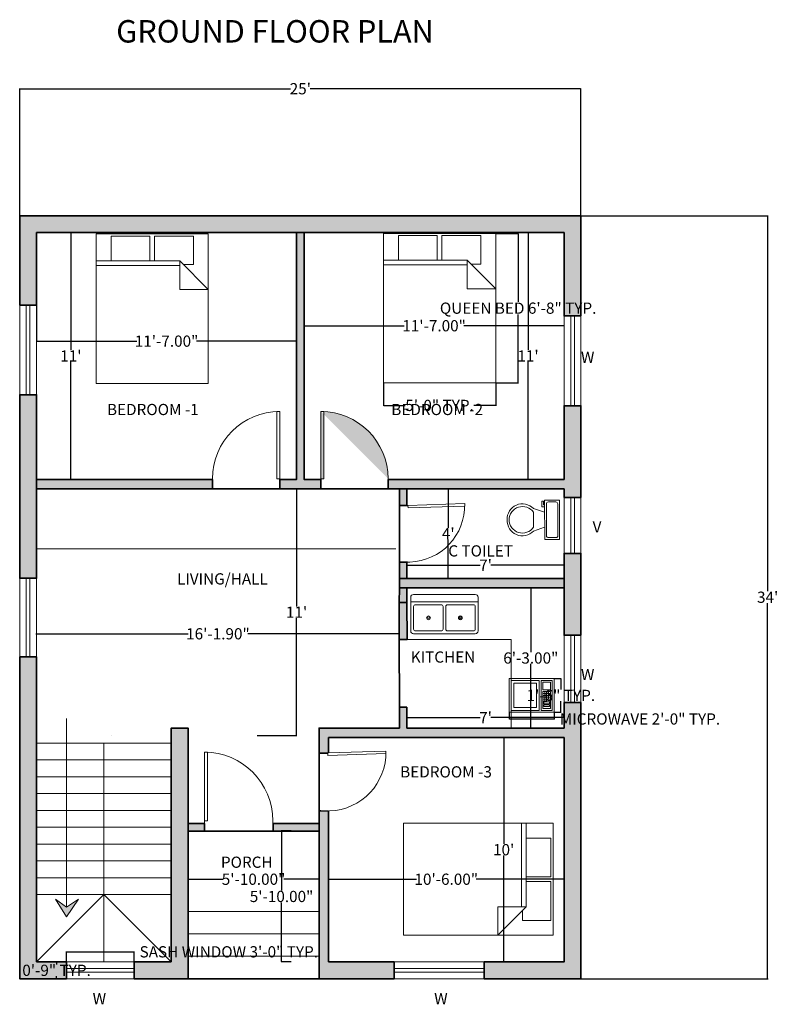
# Model space of a CAD drawing. Units: inches. Extents: x -977 to 1065, y -406 to 125.
# Tile 2 of 4: x 13 to 418, y -402 to 125. Entities that reach past the tile are written whole.
import ezdxf

# ---------------------------------------------------------------- set-up
doc = ezdxf.new("R2010")
doc.units = ezdxf.units.IN
doc.header["$MEASUREMENT"] = 0
for name, color, linetype, lineweight in [('A-ANNO-DIMS', 2, 'Continuous', 13), ('A-ANNO-TEXT', 7, 'Continuous', 18), ('A-ANNO-TITL', 7, 'Continuous', 25), ('A-AREA-IDEN', 7, 'Continuous', 18), ('A-DOOR', 3, 'Continuous', 18), ('A-EQPM', 9, 'Continuous', 18), ('A-FLOR-CASE', 8, 'Continuous', 18), ('A-FLOR-CNST', 8, 'Continuous', 13), ('A-FLOR-FIXT', 8, 'Continuous', 18), ('A-FLOR-STRS', 7, 'Continuous', 18), ('A-FURN', 8, 'Continuous', 18), ('A-GLAZ', 5, 'Continuous', 18), ('A-WALL', 7, 'Continuous', 35), ('A-WALL-PATT', 252, 'Continuous', 13)]:
    doc.layers.add(name, color=color, linetype=linetype, lineweight=lineweight)
doc.styles.get("Standard").update_dxf_attribs({"font": 'arial.ttf'})
doc.dimstyles.get("Standard").update_dxf_attribs({"dimtxt": 6, "dimasz": 0.18, "dimexe": 0.18, "dimexo": 0.0625, "dimgap": 0.09, "dimtad": 0, "dimtih": 1, "dimtoh": 1, "dimzin": 0, "dimdsep": 46, "dimlunit": 3, "dimtxsty": 'Standard', "dimcen": 0.09, "dimadec": 0, "dimazin": 0, "dimtfac": 1, "dimtofl": 0, "dimtmove": 0, "dimatfit": 3, "dimfxl": 1, "dimtolj": 1, "dimtzin": 0, "dimarcsym": 0})

# ---------------------------------------------------------------- blocks, each defined once
blk = doc.blocks.new('*U2')
for p, q in [((0, 0), (0, -6)), ((40, 0), (40, -6))]:
    blk.add_line(p, q)
blk.add_lwpolyline([(0, 0), (0, 40), (1.75, 40), (1.75, 0)], close=True)
blk.add_arc((0, 0), 40, 0, 90)
blk = doc.blocks.new('*U4')
for p, q in [((241.3, -152.4), (241.3, -50.8)), ((-254, -215.9), (-203.2, -215.9)), ((-254, -241.3), (-254, -215.9)), ((-177.8, -241.3), (-254, -241.3)), ((-203.2, -215.9), (-203.2, -203.2)), ((-177.8, -203.2), (-177.8, -241.3)), ((-101.6, -203.2), (-152.4, -355.6)), ((101.6, -203.2), (152.4, -355.6)), ((101.6, -355.6), (-101.6, -355.6))]:
    blk.add_line(p, q)
blk.add_lwpolyline([(266.7, -203.2), (266.7, 0), (-266.7, 0), (-266.7, -203.2)], close=True)
for points in [[(-241.3, -50.8), (-241.3, -152.4)], [(215.9, -25.4), (-215.9, -25.4)], [(-215.9, -177.8), (215.9, -177.8)]]:
    blk.add_lwpolyline(points)
for centre, radius, start, end in [((-219.075, -47.625), 22.45064, 81.8699, 188.1301), ((219.075, -47.625), 22.45064, 351.8699, 98.1301), ((-219.075, -155.575), 22.45064, 171.869898, 278.1301), ((219.075, -155.575), 22.45064, 261.8699, 8.1301), ((-12.12088, -505.93752), 205.61935, 133.01722, 273.38), ((0.94996, -504.77674), 181.02486, 124.50543, 269.7), ((-0.94742, -504.77674), 181.02486, 270.3, 55.4946), ((12.12342, -505.93752), 205.61935, 266.62, 46.9828)]:
    blk.add_arc(centre, radius, start, end)
blk = doc.blocks.new('Bed - Queen')
for p, q in [((0, -80.00003), (0, 0)), ((0, 0), (59.99999, 0)), ((59.99999, 0), (59.99999, -80.00003)), ((7.99999, -1.2), (28.79998, -1.2)), ((7.99999, -14.4), (7.99999, -1.2)), ((28.79998, -1.2), (28.79998, -14.4)), ((31.19999, -1.2), (51.99999, -1.2)), ((31.19999, -14.4), (31.19999, -1.2)), ((51.99999, -1.2), (51.99999, -16.4)), ((0, -14.4), (44.8, -14.4)), ((59.99999, -29.6), (44.8, -14.4)), ((44.8, -14.4), (44.8, -29.6)), ((44.8, -16.8), (0, -16.8)), ((51.99999, -16.4), (46.79936, -16.4)), ((44.8, -29.6), (59.99999, -29.6)), ((59.99999, -80.00003), (0, -80.00003))]:
    blk.add_line(p, q)
blk = doc.blocks.new('*D10')
at = {"layer": 'A-ANNO-DIMS', "color": 0, "lineweight": -2, "transparency": 16777216}
for p, q in [((35.9, 10.82), (40.14, 10.82)), ((39.96, 10.64), (39.96, -52.08)), ((39.96, -121), (39.96, -58.29)), ((35.9, -121.18), (40.14, -121.18))]:
    blk.add_line(p, q, dxfattribs=at)
at = {"layer": 'A-ANNO-DIMS', "color": 0, "transparency": 16777216}
for points in [[(39.93, 10.64), (39.99, 10.64), (39.96, 10.82)], [(39.93, -121), (39.99, -121), (39.96, -121.18)]]:
    blk.add_solid(points, dxfattribs=at)
at = {"layer": 'Defpoints', "color": 0, "transparency": 16777216}
for p in [(35.83, 10.82), (35.83, -121.18), (39.96, -121.18)]:
    blk.add_point(p, dxfattribs=at)
at = {"layer": 'A-ANNO-DIMS', "color": 0, "transparency": 16777216, "insert": (39.96, -55.18), "char_height": 6, "attachment_point": 5}
blk.add_mtext("\\A1;11'", dxfattribs=at)
blk = doc.blocks.new('*D11')
at = {"layer": 'A-ANNO-DIMS', "color": 0, "lineweight": -2, "transparency": 16777216}
for p, q in [((21.62, -17.66), (21.62, -47.42)), ((160.62, -17.66), (160.62, -47.42)), ((21.8, -47.24), (75.18, -47.24)), ((160.44, -47.24), (107.06, -47.24))]:
    blk.add_line(p, q, dxfattribs=at)
at = {"layer": 'A-ANNO-DIMS', "color": 0, "transparency": 16777216}
for points in [[(21.8, -47.21), (21.8, -47.27), (21.62, -47.24)], [(160.44, -47.21), (160.44, -47.27), (160.62, -47.24)]]:
    blk.add_solid(points, dxfattribs=at)
at = {"layer": 'Defpoints', "color": 0, "transparency": 16777216}
for p in [(21.62, -17.6), (160.62, -17.6), (160.62, -47.24)]:
    blk.add_point(p, dxfattribs=at)
at = {"layer": 'A-ANNO-DIMS', "color": 0, "transparency": 16777216, "insert": (91.12, -47.24), "char_height": 6, "attachment_point": 5}
blk.add_mtext('\\A1;11\'-7.00"', dxfattribs=at)
blk = doc.blocks.new('*D12')
at = {"layer": 'A-ANNO-DIMS', "color": 0, "lineweight": -2, "transparency": 16777216}
for p, q in [((164.62, -38.95), (164.62, -38.83)), ((164.8, -39.01), (218.18, -39.01)), ((303.44, -39.01), (250.06, -39.01)), ((303.62, -38.95), (303.62, -38.83))]:
    blk.add_line(p, q, dxfattribs=at)
at = {"layer": 'A-ANNO-DIMS', "color": 0, "transparency": 16777216}
for points in [[(164.8, -38.98), (164.8, -39.04), (164.62, -39.01)], [(303.44, -38.98), (303.44, -39.04), (303.62, -39.01)]]:
    blk.add_solid(points, dxfattribs=at)
at = {"layer": 'Defpoints', "color": 0, "transparency": 16777216}
for p in [(164.62, -39.01), (303.62, -39.01), (303.62, -39.01)]:
    blk.add_point(p, dxfattribs=at)
at = {"layer": 'A-ANNO-DIMS', "color": 0, "transparency": 16777216, "insert": (234.12, -39.01), "char_height": 6, "attachment_point": 5}
blk.add_mtext('\\A1;11\'-7.00"', dxfattribs=at)
blk = doc.blocks.new('*D13')
at = {"layer": 'A-ANNO-DIMS', "color": 0, "lineweight": -2, "transparency": 16777216}
for p, q in [((289.2, 10.82), (284.14, 10.82)), ((284.32, 10.64), (284.32, -52.08)), ((284.32, -121), (284.32, -58.29)), ((289.2, -121.18), (284.14, -121.18))]:
    blk.add_line(p, q, dxfattribs=at)
at = {"layer": 'A-ANNO-DIMS', "color": 0, "transparency": 16777216}
for points in [[(284.29, 10.64), (284.35, 10.64), (284.32, 10.82)], [(284.29, -121), (284.35, -121), (284.32, -121.18)]]:
    blk.add_solid(points, dxfattribs=at)
at = {"layer": 'Defpoints', "color": 0, "transparency": 16777216}
for p in [(289.26, 10.82), (284.32, -121.18), (289.26, -121.18)]:
    blk.add_point(p, dxfattribs=at)
at = {"layer": 'A-ANNO-DIMS', "color": 0, "transparency": 16777216, "insert": (284.32, -55.18), "char_height": 6, "attachment_point": 5}
blk.add_mtext("\\A1;11'", dxfattribs=at)
blk = doc.blocks.new('*D14')
at = {"layer": 'A-ANNO-DIMS', "color": 0, "lineweight": -2, "transparency": 16777216}
for p, q in [((261.56, -126.18), (241.51, -126.18)), ((241.69, -126.36), (241.69, -147.09)), ((241.69, -174), (241.69, -153.27)), ((261.56, -174.18), (241.51, -174.18))]:
    blk.add_line(p, q, dxfattribs=at)
at = {"layer": 'A-ANNO-DIMS', "color": 0, "transparency": 16777216}
for points in [[(241.66, -126.36), (241.72, -126.36), (241.69, -126.18)], [(241.66, -174), (241.72, -174), (241.69, -174.18)]]:
    blk.add_solid(points, dxfattribs=at)
at = {"layer": 'Defpoints', "color": 0, "transparency": 16777216}
for p in [(261.62, -126.18), (241.69, -174.18), (261.62, -174.18)]:
    blk.add_point(p, dxfattribs=at)
at = {"layer": 'A-ANNO-DIMS', "color": 0, "transparency": 16777216, "insert": (241.69, -150.18), "char_height": 6, "attachment_point": 5}
blk.add_mtext("\\A1;4'", dxfattribs=at)
blk = doc.blocks.new('*D15')
at = {"layer": 'A-ANNO-DIMS', "color": 0, "lineweight": -2, "transparency": 16777216}
for p, q in [((219.62, -169.78), (219.62, -166.89)), ((219.8, -167.07), (258.79, -167.07)), ((303.44, -167.07), (264.44, -167.07)), ((303.62, -169.78), (303.62, -166.89))]:
    blk.add_line(p, q, dxfattribs=at)
at = {"layer": 'A-ANNO-DIMS', "color": 0, "transparency": 16777216}
for points in [[(219.8, -167.04), (219.8, -167.1), (219.62, -167.07)], [(303.44, -167.04), (303.44, -167.1), (303.62, -167.07)]]:
    blk.add_solid(points, dxfattribs=at)
at = {"layer": 'Defpoints', "color": 0, "transparency": 16777216}
for p in [(303.62, -167.07), (219.62, -169.84), (303.62, -169.84)]:
    blk.add_point(p, dxfattribs=at)
at = {"layer": 'A-ANNO-DIMS', "color": 0, "transparency": 16777216, "insert": (261.62, -167.07), "char_height": 6, "attachment_point": 5}
blk.add_mtext("\\A1;7'", dxfattribs=at)
blk = doc.blocks.new('*D16')
at = {"layer": 'A-ANNO-DIMS', "color": 0, "lineweight": -2, "transparency": 16777216}
for p, q in [((219.62, -248.5), (219.62, -248.39)), ((219.8, -248.57), (258.79, -248.57)), ((303.44, -248.57), (264.44, -248.57)), ((303.62, -248.5), (303.62, -248.39))]:
    blk.add_line(p, q, dxfattribs=at)
at = {"layer": 'A-ANNO-DIMS', "color": 0, "transparency": 16777216}
for points in [[(219.8, -248.54), (219.8, -248.6), (219.62, -248.57)], [(303.44, -248.54), (303.44, -248.6), (303.62, -248.57)]]:
    blk.add_solid(points, dxfattribs=at)
at = {"layer": 'Defpoints', "color": 0, "transparency": 16777216}
for p in [(219.62, -248.57), (303.62, -248.57), (303.62, -248.57)]:
    blk.add_point(p, dxfattribs=at)
at = {"layer": 'A-ANNO-DIMS', "color": 0, "transparency": 16777216, "insert": (261.62, -248.57), "char_height": 6, "attachment_point": 5}
blk.add_mtext("\\A1;7'", dxfattribs=at)
blk = doc.blocks.new('*D17')
at = {"layer": 'A-ANNO-DIMS', "color": 0, "lineweight": -2, "transparency": 16777216}
for p, q in [((288.08, -179.18), (285.63, -179.18)), ((285.81, -179.36), (285.81, -213.53)), ((285.81, -254), (285.81, -219.84)), ((288.08, -254.18), (285.63, -254.18))]:
    blk.add_line(p, q, dxfattribs=at)
at = {"layer": 'A-ANNO-DIMS', "color": 0, "transparency": 16777216}
for points in [[(285.78, -179.36), (285.84, -179.36), (285.81, -179.18)], [(285.78, -254), (285.84, -254), (285.81, -254.18)]]:
    blk.add_solid(points, dxfattribs=at)
at = {"layer": 'Defpoints', "color": 0, "transparency": 16777216}
for p in [(288.15, -179.18), (285.81, -254.18), (288.15, -254.18)]:
    blk.add_point(p, dxfattribs=at)
at = {"layer": 'A-ANNO-DIMS', "color": 0, "transparency": 16777216, "insert": (285.81, -216.68), "char_height": 6, "attachment_point": 5}
blk.add_mtext('\\A1;6\'-3.00"', dxfattribs=at)
blk = doc.blocks.new('*D18')
at = {"layer": 'A-ANNO-DIMS', "color": 0, "lineweight": -2, "transparency": 16777216}
for p, q in [((282.32, -259.18), (271.13, -259.18)), ((271.31, -259.36), (271.31, -316.03)), ((271.31, -379), (271.31, -322.34)), ((282.15, -379.18), (271.13, -379.18))]:
    blk.add_line(p, q, dxfattribs=at)
at = {"layer": 'A-ANNO-DIMS', "color": 0, "transparency": 16777216}
for points in [[(271.28, -259.36), (271.34, -259.36), (271.31, -259.18)], [(271.28, -379), (271.34, -379), (271.31, -379.18)]]:
    blk.add_solid(points, dxfattribs=at)
at = {"layer": 'Defpoints', "color": 0, "transparency": 16777216}
for p in [(282.38, -259.18), (271.31, -379.18), (282.22, -379.18)]:
    blk.add_point(p, dxfattribs=at)
at = {"layer": 'A-ANNO-DIMS', "color": 0, "transparency": 16777216, "insert": (271.31, -319.18), "char_height": 6, "attachment_point": 5}
blk.add_mtext("\\A1;10'", dxfattribs=at)
blk = doc.blocks.new('*D19')
at = {"layer": 'A-ANNO-DIMS', "color": 0, "lineweight": -2, "transparency": 16777216}
for p, q in [((177.62, -347.23), (177.62, -334.79)), ((177.8, -334.97), (224.68, -334.97)), ((303.44, -334.97), (256.56, -334.97)), ((303.62, -343.4), (303.62, -334.79))]:
    blk.add_line(p, q, dxfattribs=at)
at = {"layer": 'A-ANNO-DIMS', "color": 0, "transparency": 16777216}
for points in [[(177.8, -334.94), (177.8, -335), (177.62, -334.97)], [(303.44, -334.94), (303.44, -335), (303.62, -334.97)]]:
    blk.add_solid(points, dxfattribs=at)
at = {"layer": 'Defpoints', "color": 0, "transparency": 16777216}
for p in [(303.62, -334.97), (177.62, -347.29), (303.62, -343.47)]:
    blk.add_point(p, dxfattribs=at)
at = {"layer": 'A-ANNO-DIMS', "color": 0, "transparency": 16777216, "insert": (240.62, -334.97), "char_height": 6, "attachment_point": 5}
blk.add_mtext('\\A1;10\'-6.00"', dxfattribs=at)
blk = doc.blocks.new('*D20')
at = {"layer": 'A-ANNO-DIMS', "color": 0, "lineweight": -2, "transparency": 16777216}
for p, q in [((102.62, -334.91), (102.62, -334.79)), ((102.8, -334.97), (121.4, -334.97)), ((172.44, -334.97), (153.84, -334.97)), ((172.62, -334.91), (172.62, -334.79))]:
    blk.add_line(p, q, dxfattribs=at)
at = {"layer": 'A-ANNO-DIMS', "color": 0, "transparency": 16777216}
for points in [[(102.8, -334.94), (102.8, -335), (102.62, -334.97)], [(172.44, -334.94), (172.44, -335), (172.62, -334.97)]]:
    blk.add_solid(points, dxfattribs=at)
at = {"layer": 'Defpoints', "color": 0, "transparency": 16777216}
for p in [(102.62, -334.97), (172.62, -334.97), (172.62, -334.97)]:
    blk.add_point(p, dxfattribs=at)
at = {"layer": 'A-ANNO-DIMS', "color": 0, "transparency": 16777216, "insert": (137.62, -334.97), "char_height": 6, "attachment_point": 5}
blk.add_mtext('\\A1;5\'-10.00"', dxfattribs=at)
blk = doc.blocks.new('*D21')
at = {"layer": 'A-ANNO-DIMS', "color": 0, "lineweight": -2, "transparency": 16777216}
for p, q in [((157.65, -309.18), (152.4, -309.18)), ((152.58, -309.36), (152.58, -341.03)), ((152.58, -379), (152.58, -347.34)), ((157.65, -379.18), (152.4, -379.18))]:
    blk.add_line(p, q, dxfattribs=at)
at = {"layer": 'A-ANNO-DIMS', "color": 0, "transparency": 16777216}
for points in [[(152.55, -309.36), (152.61, -309.36), (152.58, -309.18)], [(152.55, -379), (152.61, -379), (152.58, -379.18)]]:
    blk.add_solid(points, dxfattribs=at)
at = {"layer": 'Defpoints', "color": 0, "transparency": 16777216}
for p in [(157.72, -309.18), (152.58, -379.18), (157.72, -379.18)]:
    blk.add_point(p, dxfattribs=at)
at = {"layer": 'A-ANNO-DIMS', "color": 0, "transparency": 16777216, "insert": (152.58, -344.18), "char_height": 6, "attachment_point": 5}
blk.add_mtext('\\A1;5\'-10.00"', dxfattribs=at)
blk = doc.blocks.new('*D22')
at = {"layer": 'A-ANNO-DIMS', "color": 0, "lineweight": -2, "transparency": 16777216}
for p, q in [((139.49, -126.18), (160.8, -126.18)), ((160.62, -126.36), (160.62, -189.08)), ((160.62, -258), (160.62, -195.29)), ((139.49, -258.18), (160.8, -258.18))]:
    blk.add_line(p, q, dxfattribs=at)
at = {"layer": 'A-ANNO-DIMS', "color": 0, "transparency": 16777216}
for points in [[(160.59, -126.36), (160.65, -126.36), (160.62, -126.18)], [(160.59, -258), (160.65, -258), (160.62, -258.18)]]:
    blk.add_solid(points, dxfattribs=at)
at = {"layer": 'Defpoints', "color": 0, "transparency": 16777216}
for p in [(139.43, -126.18), (139.43, -258.18), (160.62, -258.18)]:
    blk.add_point(p, dxfattribs=at)
at = {"layer": 'A-ANNO-DIMS', "color": 0, "transparency": 16777216, "insert": (160.62, -192.18), "char_height": 6, "attachment_point": 5}
blk.add_mtext("\\A1;11'", dxfattribs=at)
blk = doc.blocks.new('*D23')
at = {"layer": 'A-ANNO-DIMS', "color": 0, "lineweight": -2, "transparency": 16777216}
for p, q in [((21.62, -204.17), (21.62, -203.55)), ((21.8, -203.73), (102.63, -203.73)), ((215.34, -203.73), (134.51, -203.73)), ((215.52, -203.66), (215.52, -203.55))]:
    blk.add_line(p, q, dxfattribs=at)
at = {"layer": 'A-ANNO-DIMS', "color": 0, "transparency": 16777216}
for points in [[(21.8, -203.7), (21.8, -203.76), (21.62, -203.73)], [(215.34, -203.7), (215.34, -203.76), (215.52, -203.73)]]:
    blk.add_solid(points, dxfattribs=at)
at = {"layer": 'Defpoints', "color": 0, "transparency": 16777216}
for p in [(21.62, -204.24), (215.52, -203.73), (215.52, -203.73)]:
    blk.add_point(p, dxfattribs=at)
at = {"layer": 'A-ANNO-DIMS', "color": 0, "transparency": 16777216, "insert": (118.57, -203.73), "char_height": 6, "attachment_point": 5}
blk.add_mtext('\\A1;16\'-1.90"', dxfattribs=at)
blk = doc.blocks.new('*D24')
at = {"layer": 'A-ANNO-DIMS', "color": 0, "lineweight": -2, "transparency": 16777216}
for p, q in [((12.62, 19.88), (12.62, 87.89)), ((12.8, 87.71), (157.39, 87.71)), ((312.44, 87.71), (167.85, 87.71)), ((312.62, 19.88), (312.62, 87.89))]:
    blk.add_line(p, q, dxfattribs=at)
at = {"layer": 'A-ANNO-DIMS', "color": 0, "transparency": 16777216}
for points in [[(12.8, 87.74), (12.8, 87.68), (12.62, 87.71)], [(312.44, 87.74), (312.44, 87.68), (312.62, 87.71)]]:
    blk.add_solid(points, dxfattribs=at)
at = {"layer": 'Defpoints', "color": 0, "transparency": 16777216}
for p in [(312.62, 87.71), (12.62, 19.82), (312.62, 19.82)]:
    blk.add_point(p, dxfattribs=at)
at = {"layer": 'A-ANNO-DIMS', "color": 0, "transparency": 16777216, "insert": (162.62, 87.71), "char_height": 6, "attachment_point": 5}
blk.add_mtext("\\A1;25'", dxfattribs=at)
blk = doc.blocks.new('*D25')
at = {"layer": 'A-ANNO-DIMS', "color": 0, "lineweight": -2, "transparency": 16777216}
for p, q in [((312.68, 19.82), (412.59, 19.82)), ((412.41, 19.64), (412.41, -181.03)), ((412.41, -388), (412.41, -187.34)), ((312.68, -388.18), (412.59, -388.18))]:
    blk.add_line(p, q, dxfattribs=at)
at = {"layer": 'A-ANNO-DIMS', "color": 0, "transparency": 16777216}
for points in [[(412.38, 19.64), (412.44, 19.64), (412.41, 19.82)], [(412.38, -388), (412.44, -388), (412.41, -388.18)]]:
    blk.add_solid(points, dxfattribs=at)
at = {"layer": 'Defpoints', "color": 0, "transparency": 16777216}
for p in [(312.62, 19.82), (312.62, -388.18), (412.41, -388.18)]:
    blk.add_point(p, dxfattribs=at)
at = {"layer": 'A-ANNO-DIMS', "color": 0, "transparency": 16777216, "insert": (412.41, -184.18), "char_height": 6, "attachment_point": 5}
blk.add_mtext("\\A1;34'", dxfattribs=at)
blk = doc.blocks.new('Microwave')
for p, q in [((19, 7), (19, 11)), ((20, 11), (20, 7)), ((21, 7), (21, 11)), ((18, 10), (22, 10)), ((22, 9), (18, 9)), ((18, 8), (22, 8)), ((22, 7), (18, 7)), ((20, 6), (18, 6)), ((19, 6), (19, 7)), ((20, 7), (20, 6))]:
    blk.add_line(p, q)
for points in [[(0, 0), (0, 18), (24, 18), (24, 0)], [(1, 1), (1, 17), (16, 17), (16, 1)], [(17, 1), (17, 17), (23, 17), (23, 1)], [(18, 12), (18, 16), (22, 16), (22, 12)], [(2.5, 2.5), (2.5, 15.5), (14.5, 15.5), (14.5, 2.5)], [(18, 2), (18, 11), (22, 11), (22, 2)], [(18.5, 4.5), (18.5, 5.5), (21.5, 5.5), (21.5, 4.5)], [(18.5, 3), (18.5, 4), (21.5, 4), (21.5, 3)]]:
    blk.add_lwpolyline(points, close=True)
blk = doc.blocks.new('Sink-double - 36 in top')
for p, q in [((-18, -4), (18, -4)), ((-0.75, -18.5), (-0.75, -6.5)), ((0.75, -6.5), (0.75, -18.5))]:
    blk.add_line(p, q)
for points in [[(-16.5, 0), (16.5, 0)], [(-18, -19.5), (-18, -1.5)], [(18, -1.5), (18, -19.5)], [(-16.5, -18.5), (-16.5, -6.5)], [(-15.5, -5.5), (-1.75, -5.5)], [(1.75, -5.5), (15.5, -5.5)], [(16.5, -6.5), (16.5, -18.5)], [(16.5, -21), (-16.5, -21)], [(-1.75, -19.5), (-15.5, -19.5)], [(15.5, -19.5), (1.75, -19.5)]]:
    blk.add_lwpolyline(points)
for centre, radius in [((-8.5, -12.5), 1), ((-8.5, -12.5), 0.5), ((8.5, -12.5), 1), ((8.5, -12.5), 0.5)]:
    blk.add_circle(centre, radius)
for centre, radius, start, end in [((-16.5, -1.5), 1.5, 90, 180), ((16.5, -1.5), 1.5, 0, 90), ((-15.5, -6.5), 1, 90, 180), ((-1.75, -6.5), 1, 0, 90), ((1.75, -6.5), 1, 90, 180), ((15.5, -6.5), 1, 0, 90), ((-16.5, -19.5), 1.5, 180, 270), ((-15.5, -18.5), 1, 180, 270), ((-1.75, -18.5), 1, 270, 0), ((1.75, -18.5), 1, 180, 270), ((15.5, -18.5), 1, 270, 0), ((16.5, -19.5), 1.5, 270, 0)]:
    blk.add_arc(centre, radius, start, end)
blk = doc.blocks.new('WIN-48-FRAMED')
for p, q in [((0, 48), (9, 48)), ((0, 0), (0, 48)), ((3.5, 0), (3.5, 48)), ((5.5, 48), (5.5, 0)), ((9, 48), (9, 0)), ((9, 0), (0, 0))]:
    blk.add_line(p, q)
for points in [[(0, 0), (0, 48)], [(9, 0), (9, 48)]]:
    blk.add_lwpolyline(points)
blk = doc.blocks.new('WIN-48-SASH')
for p, q in [((48, 9), (0, 9)), ((48, 5.5), (0, 5.5)), ((0, 3.5), (48, 3.5)), ((0, 0), (48, 0))]:
    blk.add_line(p, q)
for points in [[(48, 9), (0, 9)], [(48, 0), (0, 0)]]:
    blk.add_lwpolyline(points)
blk = doc.blocks.new('WIN-36-SASH')
for p, q in [((36, 9), (0, 9)), ((36, 5.5), (0, 5.5)), ((0, 3.5), (36, 3.5)), ((0, 0), (36, 0))]:
    blk.add_line(p, q)
for points in [[(36, 9), (0, 9)], [(36, 0), (0, 0)]]:
    blk.add_lwpolyline(points)
blk = doc.blocks.new('*D50')
at = {"layer": 'A-ANNO-DIMS', "color": 0, "lineweight": -2, "transparency": 16777216}
for p, q in [((267.1, 10.39), (279.22, 10.39)), ((279.04, 10.21), (279.04, -26.23)), ((279.04, -69.43), (279.04, -32.99)), ((267.1, -69.61), (279.22, -69.61))]:
    blk.add_line(p, q, dxfattribs=at)
at = {"layer": 'A-ANNO-DIMS', "color": 0, "transparency": 16777216}
for points in [[(279.01, 10.21), (279.07, 10.21), (279.04, 10.39)], [(279.01, -69.43), (279.07, -69.43), (279.04, -69.61)]]:
    blk.add_solid(points, dxfattribs=at)
at = {"layer": 'Defpoints', "color": 0, "transparency": 16777216}
for p in [(267.04, 10.39), (279.04, 10.39), (267.04, -69.61)]:
    blk.add_point(p, dxfattribs=at)
at = {"layer": 'A-ANNO-DIMS', "color": 0, "transparency": 16777216, "insert": (279.04, -29.61), "char_height": 6, "attachment_point": 5}
blk.add_mtext('\\A1;QUEEN BED 6\'-8" TYP.', dxfattribs=at)
blk = doc.blocks.new('*D51')
at = {"layer": 'A-ANNO-DIMS', "color": 0, "lineweight": -2, "transparency": 16777216}
for p, q in [((207.04, -69.67), (207.04, -81.79)), ((267.04, -69.67), (267.04, -81.79)), ((207.22, -81.61), (218.66, -81.61)), ((266.86, -81.61), (255.41, -81.61))]:
    blk.add_line(p, q, dxfattribs=at)
at = {"layer": 'A-ANNO-DIMS', "color": 0, "transparency": 16777216}
for points in [[(207.22, -81.58), (207.22, -81.64), (207.04, -81.61)], [(266.86, -81.58), (266.86, -81.64), (267.04, -81.61)]]:
    blk.add_solid(points, dxfattribs=at)
at = {"layer": 'Defpoints', "color": 0, "transparency": 16777216}
for p in [(207.04, -69.61), (267.04, -69.61), (267.04, -81.61)]:
    blk.add_point(p, dxfattribs=at)
at = {"layer": 'A-ANNO-DIMS', "color": 0, "transparency": 16777216, "insert": (237.04, -81.61), "char_height": 6, "attachment_point": 5}
blk.add_mtext('\\A1;5\'-0" TYP.', dxfattribs=at)
blk = doc.blocks.new('*D62')
at = {"layer": 'A-ANNO-DIMS', "color": 0, "lineweight": -2, "transparency": 16777216}
for p, q in [((274.27, -245.74), (274.27, -249.46)), ((298.27, -245.74), (298.27, -249.46)), ((274.45, -249.28), (298.09, -249.28)), ((298.27, -249.28), (298.45, -249.28))]:
    blk.add_line(p, q, dxfattribs=at)
at = {"layer": 'A-ANNO-DIMS', "color": 0, "transparency": 16777216}
for points in [[(274.45, -249.25), (274.45, -249.31), (274.27, -249.28)], [(298.09, -249.25), (298.09, -249.31), (298.27, -249.28)]]:
    blk.add_solid(points, dxfattribs=at)
at = {"layer": 'Defpoints', "color": 0, "transparency": 16777216}
for p in [(274.27, -245.68), (298.27, -245.68), (298.27, -249.28)]:
    blk.add_point(p, dxfattribs=at)
at = {"layer": 'A-ANNO-DIMS', "color": 0, "transparency": 16777216, "insert": (344.16, -249.28), "char_height": 6, "attachment_point": 5}
blk.add_mtext('\\A1;MICROWAVE 2\'-0" TYP.', dxfattribs=at)
blk = doc.blocks.new('*D63')
at = {"layer": 'A-ANNO-DIMS', "color": 0, "lineweight": -2, "transparency": 16777216}
for p, q in [((298.33, -227.68), (302.05, -227.68)), ((301.87, -227.86), (301.87, -233.52)), ((301.87, -245.5), (301.87, -239.83)), ((298.33, -245.68), (302.05, -245.68))]:
    blk.add_line(p, q, dxfattribs=at)
at = {"layer": 'A-ANNO-DIMS', "color": 0, "transparency": 16777216}
for points in [[(301.84, -227.86), (301.9, -227.86), (301.87, -227.68)], [(301.84, -245.5), (301.9, -245.5), (301.87, -245.68)]]:
    blk.add_solid(points, dxfattribs=at)
at = {"layer": 'Defpoints', "color": 0, "transparency": 16777216}
for p in [(298.27, -227.68), (301.87, -227.68), (298.27, -245.68)]:
    blk.add_point(p, dxfattribs=at)
at = {"layer": 'A-ANNO-DIMS', "color": 0, "transparency": 16777216, "insert": (301.87, -236.68), "char_height": 6, "attachment_point": 5}
blk.add_mtext('\\A1;1\'-6" TYP.', dxfattribs=at)
blk = doc.blocks.new('*D64')
at = {"layer": 'A-ANNO-DIMS', "color": 0, "lineweight": -2, "transparency": 16777216}
for p, q in [((37.72, -379.12), (37.72, -373.6)), ((37.9, -373.78), (73.54, -373.78)), ((73.72, -379.12), (73.72, -373.6)), ((73.72, -373.78), (73.9, -373.78))]:
    blk.add_line(p, q, dxfattribs=at)
at = {"layer": 'A-ANNO-DIMS', "color": 0, "transparency": 16777216}
for points in [[(37.9, -373.75), (37.9, -373.81), (37.72, -373.78)], [(73.54, -373.75), (73.54, -373.81), (73.72, -373.78)]]:
    blk.add_solid(points, dxfattribs=at)
at = {"layer": 'Defpoints', "color": 0, "transparency": 16777216}
for p in [(73.72, -373.78), (37.72, -379.18), (73.72, -379.18)]:
    blk.add_point(p, dxfattribs=at)
at = {"layer": 'A-ANNO-DIMS', "color": 0, "transparency": 16777216, "insert": (124.39, -373.78), "char_height": 6, "attachment_point": 5}
blk.add_mtext('\\A1;SASH WINDOW 3\'-0" TYP.', dxfattribs=at)
blk = doc.blocks.new('*D65')
at = {"layer": 'A-ANNO-DIMS', "color": 0, "lineweight": -2, "transparency": 16777216}
for p, q in [((37.65, -379.18), (32.14, -379.18)), ((32.32, -379.36), (32.32, -380.53)), ((37.65, -388.18), (32.14, -388.18)), ((32.32, -388), (32.32, -386.84))]:
    blk.add_line(p, q, dxfattribs=at)
at = {"layer": 'A-ANNO-DIMS', "color": 0, "transparency": 16777216}
for points in [[(32.29, -379.36), (32.35, -379.36), (32.32, -379.18)], [(32.29, -388), (32.35, -388), (32.32, -388.18)]]:
    blk.add_solid(points, dxfattribs=at)
at = {"layer": 'Defpoints', "color": 0, "transparency": 16777216}
for p in [(32.32, -379.18), (37.72, -379.18), (37.72, -388.18)]:
    blk.add_point(p, dxfattribs=at)
at = {"layer": 'A-ANNO-DIMS', "color": 0, "transparency": 16777216, "insert": (32.32, -383.68), "char_height": 6, "attachment_point": 5}
blk.add_mtext('\\A1;0\'-9" TYP.', dxfattribs=at)

msp = doc.modelspace()

# ---------------------------------------------------------------- hatches: boundary and pattern name
at = {"layer": 'A-FLOR-STRS'}
h = msp.add_hatch(color=256, dxfattribs=at)
h.dxf.hatch_style = 1
h.paths.add_polyline_path([(43.997, -345.721), (37.705, -355.048), (31.71, -345.721), (37.705, -349.917)])
at = {"layer": 'A-WALL-PATT'}
h = msp.add_hatch(color=256, dxfattribs=at)
h.dxf.hatch_style = 1
h.paths.add_polyline_path([(312.619, -33.787), (312.619, 19.815), (12.619, 19.815), (12.619, -27.943), (21.619, -27.943), (21.619, 10.815), (303.619, 10.815), (303.619, -33.787)])
h = msp.add_hatch(color=256, dxfattribs=at)
h.dxf.hatch_style = 1
h.paths.add_polyline_path([(173.619, -126.185), (151.619, -126.185), (151.619, -121.185), (160.619, -121.185), (160.619, 10.815), (164.619, 10.815), (164.619, -121.185), (173.619, -121.185)])
h = msp.add_hatch(color=256, dxfattribs=at)
h.dxf.hatch_style = 1
h.paths.add_polyline_path([(21.619, -126.185), (21.619, -174.067), (12.619, -174.067), (12.619, -75.943), (21.619, -75.943), (21.619, -121.185)])
h.paths.add_polyline_path([(21.619, -379.185), (37.717, -379.185), (37.717, -388.185), (12.619, -388.185), (12.619, -334.185), (12.619, -216.067), (21.619, -216.067)])
h.paths.add_polyline_path([(260.813, -388.185), (312.619, -388.185), (312.619, -240.505), (303.619, -240.505), (303.619, -379.185), (260.813, -379.185)])
h.paths.add_polyline_path([(312.619, -204.505), (312.619, -160.768), (303.619, -160.768), (303.619, -204.505)])
edge = h.paths.add_edge_path()
edge.add_line((312.619, -81.787), (303.619, -81.787))
edge.add_line((303.619, -81.787), (303.619, -126.185))
h.paths.add_polyline_path([(102.619, -388.185), (102.619, -379.185), (73.717, -379.185), (73.717, -388.185)])
h.paths.add_polyline_path([(172.619, -379.185), (172.619, -388.185), (212.813, -388.185), (212.813, -379.185)])
h = msp.add_hatch(color=256, dxfattribs=at)
h.dxf.hatch_style = 1
h.paths.add_polyline_path([(303.619, -126.185), (303.619, -130.768), (312.619, -130.768), (312.619, -81.787), (303.619, -81.787), (303.619, -121.185)])
h = msp.add_hatch(color=256, dxfattribs=at)
h.dxf.hatch_style = 1
h.paths.add_polyline_path([(173.619, -120.799), (173.619, -84.891), (175.189, -84.891), (175.189, -120.799)], flags=16)
edge = h.paths.add_edge_path()
edge.add_arc((173.619, -120.799), 35.908, 0, 90)
edge = h.paths.add_edge_path()
edge.add_line((173.619, -120.799), (173.619, -126.185))
edge = h.paths.add_edge_path()
edge.add_line((209.526, -120.799), (209.526, -126.185))
edge = h.paths.add_edge_path()
edge.add_line((215.619, -126.185), (219.619, -126.185))
edge.add_line((219.619, -126.185), (303.619, -126.185))
edge.add_line((303.619, -126.185), (303.619, -121.185))
edge.add_line((303.619, -121.185), (209.526, -121.185))
edge.add_line((209.619, -121.185), (209.526, -126.185))
edge.add_line((209.526, -126.185), (215.591, -126.185))
h = msp.add_hatch(color=256, dxfattribs=at)
h.dxf.hatch_style = 1
h.paths.add_polyline_path([(21.619, -121.185), (115.666, -121.185), (115.619, -126.185), (21.619, -126.185)])
h = msp.add_hatch(color=256, dxfattribs=at)
h.dxf.hatch_style = 1
h.paths.add_polyline_path([(209.619, -126.185), (219.619, -126.185), (303.619, -126.185), (303.619, -121.185), (209.619, -121.185)])
h = msp.add_hatch(color=256, dxfattribs=at)
h.dxf.hatch_style = 1
h.paths.add_polyline_path([(215.619, -126.185), (215.619, -135.185), (215.751, -135.185), (219.619, -135.185), (219.619, -126.185)])
h = msp.add_hatch(color=256, dxfattribs=at)
h.dxf.hatch_style = 1
h.paths.add_polyline_path([(215.619, -174.185), (219.619, -174.185), (219.619, -165.504), (215.619, -165.504)])
h = msp.add_hatch(color=256, dxfattribs=at)
h.dxf.hatch_style = 1
h.paths.add_polyline_path([(303.619, -179.185), (303.619, -174.185), (215.619, -174.185), (215.619, -179.185)])
h = msp.add_hatch(color=256, dxfattribs=at)
h.dxf.hatch_style = 1
h.paths.add_polyline_path([(215.619, -187.076), (219.619, -187.076), (219.619, -179.185), (215.619, -179.185)])
h.paths.add_polyline_path([(219.619, -242.949), (215.619, -242.949), (215.619, -254.185), (177.619, -254.185), (177.619, -259.185), (303.619, -259.185), (303.619, -254.185), (219.619, -254.185)])
h = msp.add_hatch(color=256, dxfattribs=at)
h.dxf.hatch_style = 1
h.paths.add_polyline_path([(215.523, -206.737), (215.471, -187.076), (219.619, -187.076), (219.67, -206.726)])
h = msp.add_hatch(color=256, dxfattribs=at)
h.dxf.hatch_style = 1
h.paths.add_polyline_path([(102.619, -305.185), (102.619, -254.185), (93.619, -254.185), (93.619, -379.185), (102.619, -379.185), (102.619, -309.185)])
h = msp.add_hatch(color=256, dxfattribs=at)
h.dxf.hatch_style = 1
h.paths.add_polyline_path([(172.619, -267.509), (177.619, -267.36), (177.619, -254.185), (172.619, -254.185)])
h = msp.add_hatch(color=256, dxfattribs=at)
h.dxf.hatch_style = 1
h.paths.add_polyline_path([(172.619, -298.475), (172.619, -379.185), (177.619, -379.185), (177.619, -298.536)])
h = msp.add_hatch(color=256, dxfattribs=at)
h.dxf.hatch_style = 1
h.paths.add_polyline_path([(111.315, -305.185), (102.619, -305.185), (102.619, -309.185), (111.315, -309.185)])
h = msp.add_hatch(color=256, dxfattribs=at)
h.dxf.hatch_style = 1
h.paths.add_polyline_path([(172.619, -309.185), (172.619, -305.185), (148.01, -305.185), (148.01, -309.185)])

# ---------------------------------------------------------------- linework, layer by layer
at = {"layer": 'A-FLOR-CASE'}
for p, q in [((220.546, -206.724), (219.67, -206.726)), ((220.546, -206.724), (275.27, -206.724)), ((275.27, -206.724), (275.27, -254.185))]:
    msp.add_line(p, q, dxfattribs=at)
at = {"layer": 'A-FLOR-CNST'}
for p, q in [((21.619, -158.24), (213.619, -158.24)), ((61.812, -258.185), (61.812, -258.185))]:
    msp.add_line(p, q, dxfattribs=at)
at = {"layer": 'A-FLOR-STRS'}
for p, q in [((37.705, -248.978), (37.705, -349.917)), ((57.619, -262.185), (57.619, -379.185)), ((21.619, -379.185), (57.619, -343.185)), ((31.71, -345.721), (37.705, -355.048)), ((31.71, -345.721), (37.705, -349.917)), ((37.705, -349.917), (37.705, -345.721)), ((43.997, -345.721), (37.705, -355.048)), ((37.705, -349.917), (37.705, -345.721)), ((37.705, -349.917), (43.997, -345.721)), ((57.619, -343.185), (93.619, -379.185)), ((37.705, -355.048), (37.705, -355.048))]:
    msp.add_line(p, q, dxfattribs=at)
for points in [[(93.619, -262.185), (21.619, -262.185)], [(93.619, -271.185), (21.619, -271.185)], [(93.619, -280.185), (21.619, -280.185)], [(93.619, -289.185), (21.619, -289.185)], [(93.619, -298.185), (21.619, -298.185)], [(93.619, -307.185), (21.619, -307.185)], [(93.619, -316.185), (21.619, -316.185)], [(93.619, -325.185), (21.619, -325.185)], [(93.619, -334.185), (21.619, -334.185)], [(93.619, -343.185), (21.619, -343.185)], [(102.619, -352.185), (172.619, -352.185)], [(102.619, -364.185), (172.619, -364.185)], [(102.619, -376.185), (172.619, -376.185)]]:
    msp.add_lwpolyline(points, dxfattribs=at)
at = {"layer": 'A-GLAZ'}
for p, q in [((312.619, -33.787), (303.619, -33.787)), ((303.619, -33.787), (303.619, -81.787)), ((307.119, -33.787), (307.119, -81.787)), ((309.119, -81.787), (309.119, -33.787)), ((312.619, -81.787), (312.619, -33.787)), ((303.619, -130.768), (303.619, -160.768)), ((307.119, -130.768), (307.119, -160.768)), ((309.119, -160.768), (309.119, -130.768)), ((312.619, -160.768), (312.619, -130.768)), ((21.619, -174.067), (12.619, -174.067)), ((12.619, -174.067), (12.619, -216.067)), ((16.119, -174.067), (16.119, -216.067)), ((18.119, -216.067), (18.119, -174.067))]:
    msp.add_line(p, q, dxfattribs=at)
for points in [[(303.619, -33.787), (303.619, -81.787)], [(312.619, -33.787), (312.619, -82.278)], [(303.619, -130.768), (303.619, -160.768)], [(312.619, -130.768), (312.619, -160.768)], [(12.619, -216.067), (12.619, -174.067)], [(21.619, -216.067), (21.619, -174.067)], [(303.619, -240.505), (312.619, -240.505)]]:
    msp.add_lwpolyline(points, dxfattribs=at)
at = {"layer": 'A-WALL'}
for p, q in [((115.614, -121.185), (115.666, -121.185)), ((151.619, -121.185), (151.619, -126.185)), ((173.619, -121.185), (173.619, -126.185)), ((215.619, -126.185), (215.619, -165.504)), ((215.619, -165.185), (215.619, -165.185)), ((219.619, -165.185), (219.619, -165.108)), ((215.619, -179.185), (215.471, -187.076)), ((219.619, -187.076), (219.619, -179.185)), ((215.471, -187.076), (219.619, -187.076)), ((215.619, -242.949), (215.523, -206.737)), ((215.619, -242.949), (219.619, -242.949)), ((172.619, -254.185), (172.619, -298.385)), ((173.516, -298.385), (172.619, -298.385)), ((111.315, -309.185), (111.619, -309.185)), ((102.619, -379.185), (102.619, -388.185)), ((172.619, -379.185), (172.619, -388.185))]:
    msp.add_line(p, q, dxfattribs=at)
for points in [[(312.619, -33.787), (312.619, 19.815), (12.619, 19.815), (12.619, -27.943), (21.619, -27.943), (21.619, 10.815), (160.619, 10.815)], [(164.619, 10.815), (303.619, 10.815), (303.619, -33.787), (312.619, -33.787)], [(303.619, -126.185), (303.619, -130.768), (312.619, -130.768), (312.619, -81.787), (303.619, -81.787), (303.619, -121.185)], [(21.619, -121.185), (115.666, -121.185), (115.619, -126.185), (21.619, -126.185)], [(115.619, -126.185), (173.619, -126.185)], [(151.619, -121.185), (160.619, -121.185)], [(164.619, -121.185), (173.619, -121.185)], [(173.619, -126.185), (215.619, -126.185)], [(303.619, -121.185), (209.619, -121.185), (209.619, -126.185)], [(209.619, -126.185), (215.619, -126.185)], [(209.619, -126.185), (219.619, -126.185)], [(215.591, -126.185), (215.619, -126.185), (215.619, -135.185), (215.751, -135.185), (219.619, -135.185), (219.619, -126.185), (215.619, -126.185)], [(219.619, -126.185), (303.619, -126.185)], [(215.619, -135.185), (215.619, -165.268)], [(312.619, -204.505), (312.619, -160.768), (303.619, -160.768), (303.619, -174.185)], [(215.619, -165.268), (215.619, -165.504)], [(215.619, -174.204), (215.619, -174.185), (219.619, -174.185), (219.619, -165.504), (215.619, -165.504), (215.619, -174.185)], [(215.619, -174.204), (215.619, -179.185)], [(303.619, -179.185), (303.619, -174.185), (219.619, -174.185)], [(219.619, -187.076), (219.619, -179.185), (215.619, -179.185)], [(219.619, -179.185), (303.619, -179.185)], [(303.619, -179.185), (303.619, -204.505), (312.619, -204.505)], [(219.619, -187.076), (219.67, -206.726), (215.523, -206.737), (215.471, -187.076)], [(260.813, -388.185), (312.619, -388.185), (312.619, -240.505), (303.619, -240.505), (303.619, -254.185)], [(215.619, -242.949), (215.619, -254.185), (177.619, -254.185)], [(303.619, -254.185), (219.619, -254.185), (219.619, -242.949)], [(102.619, -305.185), (102.619, -254.185), (93.619, -254.185), (93.619, -379.185)], [(177.281, -267.509), (172.619, -267.509), (172.619, -254.185), (177.619, -254.185)], [(177.619, -259.185), (177.619, -267.36)], [(177.619, -259.185), (303.619, -259.185)], [(303.619, -259.185), (303.619, -379.185), (260.813, -379.185), (260.813, -388.185)], [(173.516, -298.385), (172.619, -298.385), (172.619, -298.475)], [(172.619, -298.475), (172.619, -305.185)], [(177.619, -379.185), (177.619, -298.536), (172.619, -298.475)], [(177.619, -298.385), (177.611, -298.385)], [(177.619, -298.263), (177.619, -298.263)], [(102.619, -309.185), (111.315, -309.185), (111.315, -305.185)], [(102.619, -379.185), (102.619, -309.185), (102.619, -305.185), (102.644, -305.185)], [(111.315, -305.185), (102.644, -305.185)], [(147.948, -309.185), (102.619, -309.185)], [(172.619, -309.185), (172.619, -379.185)], [(93.619, -379.185), (73.717, -379.185), (73.717, -388.185), (212.813, -388.185), (212.813, -379.185)], [(212.813, -379.185), (177.619, -379.185)]]:
    msp.add_lwpolyline(points, dxfattribs=at)
for points in [[(173.619, -126.185), (151.619, -126.185), (151.619, -121.185), (160.619, -121.185), (160.619, 10.815), (164.619, 10.815), (164.619, -121.185), (173.619, -121.185)], [(21.619, -126.185), (21.619, -174.067), (12.619, -174.067), (12.619, -75.943), (21.619, -75.943), (21.619, -121.185)], [(21.619, -379.185), (37.717, -379.185), (37.717, -388.185), (12.619, -388.185), (12.619, -334.185), (12.619, -216.067), (21.619, -216.067)], [(172.619, -309.185), (172.619, -305.185), (148.01, -305.185), (148.01, -309.185)]]:
    msp.add_lwpolyline(points, close=True, dxfattribs=at)

# ---------------------------------------------------------------- block references
at = {"layer": 'A-DOOR'}
for p, xscale, yscale, zscale in [((151.619, -120.792), -0.8988107345155221, 0.8988107345155221, 0.8988107345155221), ((173.619, -120.799), 0.8976985381560085, 0.8976985381560085, 0.8976985381560085), ((111.311, -303.689), 0.9159253945661985, 0.9159253945661985, 0.9159253945661985)]:
    msp.add_blockref('*U2', p, dxfattribs=dict(at, xscale=xscale, yscale=yscale, zscale=zscale))
at = {"layer": 'A-DOOR', "rotation": 271.702481617009}
for p, xscale, yscale, zscale in [((220.164, -135.05), 0.758190939253547, 0.758190939253547, 0.758190939253547), ((177.277, -267.37), 0.7766777877215418, 0.7766777877215418, 0.7766777877215418)]:
    msp.add_blockref('*U2', p, dxfattribs=dict(at, xscale=xscale, yscale=yscale, zscale=zscale))
at = {"layer": 'A-EQPM'}
msp.add_blockref('Microwave', (274.27, -245.675), dxfattribs=at)
at = {"layer": 'A-FLOR-FIXT', "xscale": 0.0393700787401575, "yscale": 0.0393700787401575, "zscale": 0.0393700787401575, "rotation": 270.1478125152553}
msp.add_blockref('*U4', (301.202, -142.738), dxfattribs=at)
at = {"layer": 'A-FLOR-FIXT'}
msp.add_blockref('Sink-double - 36 in top', (239.64, -182.695), dxfattribs=at)
at = {"layer": 'A-FURN'}
for p in [(53.431, 10.045), (207.035, 10.389)]:
    msp.add_blockref('Bed - Queen', p, dxfattribs=at)
at = {"layer": 'A-FURN', "rotation": 270}
msp.add_blockref('Bed - Queen', (297.699, -304.969), dxfattribs=at)
at = {"layer": 'A-GLAZ'}
for name, p in [('WIN-48-FRAMED', (12.619, -75.943)), ('WIN-36-SASH', (37.717, -388.185)), ('WIN-48-SASH', (212.813, -388.185))]:
    msp.add_blockref(name, p, dxfattribs=at)
at = {"layer": 'A-GLAZ', "rotation": 89.99999999999999}
msp.add_blockref('WIN-36-SASH', (312.619, -240.505), dxfattribs=at)

# ---------------------------------------------------------------- texts
at = {"layer": 'A-ANNO-TEXT', "char_height": 6, "attachment_point": 1}
for s, insert in [('W ', (312.619, -52.862)), ('V ', (318.851, -143.568)), ('W ', (312.619, -222.505)), ('W ', (51.61, -395.852)), ('W ', (234.174, -395.852))]:
    msp.add_mtext_dynamic_manual_height_columns(s, width=77.77408, gutter_width=1, heights=[0], dxfattribs=dict(at, insert=insert))
at = {"layer": 'A-ANNO-TITL', "insert": (64.21, 124.419), "char_height": 12, "attachment_point": 1}
msp.add_mtext_dynamic_manual_height_columns('GROUND FLOOR PLAN ', width=255.23349, gutter_width=1, heights=[0], dxfattribs=at)
at = {"layer": 'A-AREA-IDEN', "char_height": 6, "attachment_point": 1}
for s, insert in [('BEDROOM -1', (59.266, -80.799)), ('BEDROOM -2', (211.223, -80.799)), ('C TOILET ', (241.685, -156.418)), ('LIVING/HALL ', (96.691, -171.382)), ('KITCHEN', (221.635, -213.168)), ('BEDROOM -3', (215.974, -274.559)), ('PORCH', (120.163, -322.876))]:
    msp.add_mtext_dynamic_manual_height_columns(s, width=77.77408, gutter_width=1, heights=[0], dxfattribs=dict(at, insert=insert))

# ---------------------------------------------------------------- dimensions: what is measured, and where the dimension line sits
at = {"layer": 'A-ANNO-DIMS'}
for base, p1, p2, picture, middle in [((312.619, 87.715), (12.619, 19.815), (312.619, 19.815), '*D24', (162.619, 87.715)), ((160.619, -47.245), (21.619, -17.598), (160.619, -17.598), '*D11', (91.119, -47.245)), ((303.619, -39.009), (164.619, -39.009), (303.619, -39.009), '*D12', (234.119, -39.009)), ((303.619, -167.066), (219.619, -169.845), (303.619, -169.845), '*D15', (261.619, -167.066)), ((215.515, -203.726), (21.619, -204.237), (215.515, -203.726), '*D23', (118.567, -203.726)), ((303.619, -248.567), (219.619, -248.567), (303.619, -248.567), '*D16', (261.619, -248.567)), ((172.619, -334.969), (102.619, -334.969), (172.619, -334.969), '*D20', (137.619, -334.969)), ((303.619, -334.969), (177.619, -347.293), (303.619, -343.466), '*D19', (240.619, -334.969))]:
    dim = msp.add_linear_dim(base=base, p1=p1, p2=p2, dimstyle='Standard', override={"dimclrd": 0, "dimclre": 0, "dimclrt": 0}, dxfattribs=at)
    dim.commit()
    dim.dimension.update_dxf_attribs({"geometry": picture, "text_midpoint": middle})
for base, p1, p2, picture, middle in [((412.413, -388.185), (312.619, 19.815), (312.619, -388.185), '*D25', (412.413, -184.185)), ((39.955, -121.185), (35.834, 10.815), (35.834, -121.185), '*D10', (39.955, -55.185)), ((284.319, -121.185), (289.264, 10.815), (289.264, -121.185), '*D13', (284.319, -55.185)), ((160.62, -258.185), (139.431, -126.185), (139.431, -258.185), '*D22', (160.62, -192.185)), ((241.685, -174.185), (261.619, -126.185), (261.619, -174.185), '*D14', (241.685, -150.185)), ((285.814, -254.185), (288.147, -179.185), (288.147, -254.185), '*D17', (285.814, -216.685)), ((271.313, -379.185), (282.378, -259.185), (282.216, -379.185), '*D18', (271.313, -319.185)), ((152.579, -379.185), (157.716, -309.185), (157.716, -379.185), '*D21', (152.579, -344.185))]:
    dim = msp.add_linear_dim(base=base, p1=p1, p2=p2, angle=90, dimstyle='Standard', override={"dimclrd": 0, "dimclre": 0, "dimclrt": 0}, dxfattribs=at)
    dim.commit()
    dim.dimension.update_dxf_attribs({"geometry": picture, "text_midpoint": middle})
for base, p1, p2, text, picture, middle in [((279.035, 10.389), (267.035, -69.611), (267.035, 10.389), 'QUEEN BED <> TYP.', '*D50', (279.035, -29.611)), ((301.87, -227.675), (298.27, -245.675), (298.27, -227.675), '<> TYP.', '*D63', (301.87, -236.675)), ((32.317, -379.185), (37.717, -388.185), (37.717, -379.185), '<> TYP.', '*D65', (32.317, -383.685))]:
    dim = msp.add_linear_dim(base=base, p1=p1, p2=p2, angle=90, text=text, dimstyle='Standard', override={"dimdec": 1, "dimlfac": 1, "dimrnd": 0, "dimzin": 1, "dimdsep": 46, "dimlunit": 4, "dimfrac": 2}, dxfattribs=at)
    dim.commit()
    dim.dimension.update_dxf_attribs({"geometry": picture, "text_midpoint": middle})
for base, p1, p2, text, picture, middle in [((267.035, -81.611), (207.035, -69.611), (267.035, -69.611), '<> TYP.', '*D51', (237.035, -81.611)), ((298.27, -249.275), (274.27, -245.675), (298.27, -245.675), 'MICROWAVE <> TYP.', '*D62', (344.164, -249.275)), ((73.717, -373.785), (37.717, -379.185), (73.717, -379.185), 'SASH WINDOW <> TYP.', '*D64', (124.39, -373.785))]:
    dim = msp.add_linear_dim(base=base, p1=p1, p2=p2, text=text, dimstyle='Standard', override={"dimdec": 1, "dimlfac": 1, "dimrnd": 0, "dimzin": 1, "dimdsep": 46, "dimlunit": 4, "dimfrac": 2}, dxfattribs=at)
    dim.commit()
    dim.dimension.update_dxf_attribs({"geometry": picture, "text_midpoint": middle})

doc.saveas('drawing.dxf')
